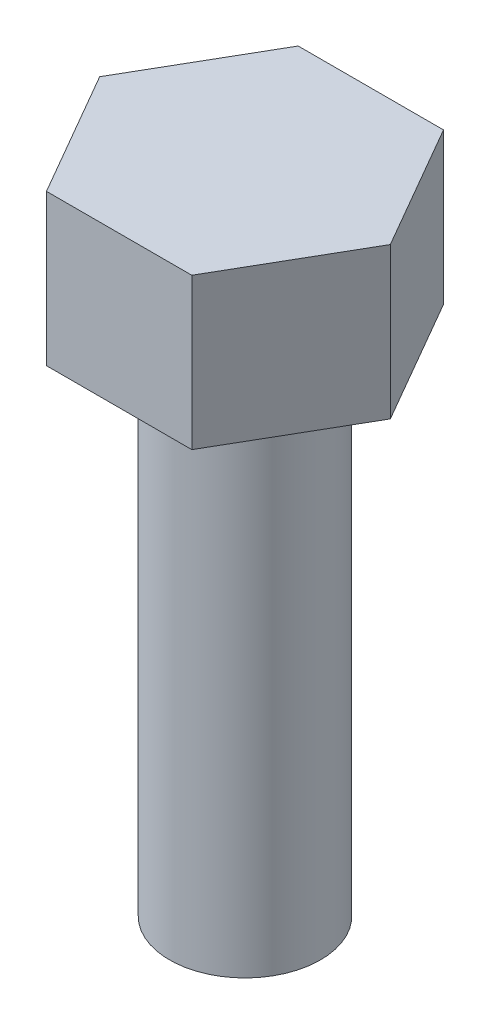
from build123d import *

# Parameters (mm, degrees)
HEX_HEAD_5AF_X_3_DEPTH = 3
SHANK_PROFILE_3_R      = 1.5
SHANK_3_X_10_DEPTH     = 10


with BuildPart() as part:
    # Hex Head Profile → Hex Head 5AF x 3 (new body)
    with BuildSketch(Plane(origin=(0, 0, 0), x_dir=(1, 0, 0), z_dir=(0, 1, 0))):
        Polygon((2.886751346, 0), (1.443375673, 2.5), (-1.443375673, 2.5), (-2.886751346, 0), (-1.443375673, -2.5), (1.443375673, -2.5), align=None)
    extrude(amount=HEX_HEAD_5AF_X_3_DEPTH)

    # Shank Profile Ø3 → Shank Ø3 x 10 (add)
    with BuildSketch(Plane.XZ):
        with Locations(Location((0, 0, 0), (0, 0, 270))):
            Circle(SHANK_PROFILE_3_R)
    extrude(amount=SHANK_3_X_10_DEPTH)


solid = part.part
